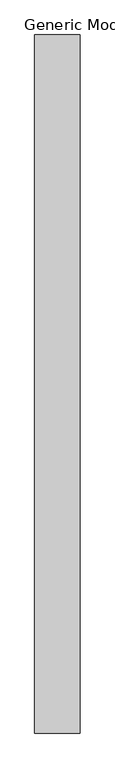
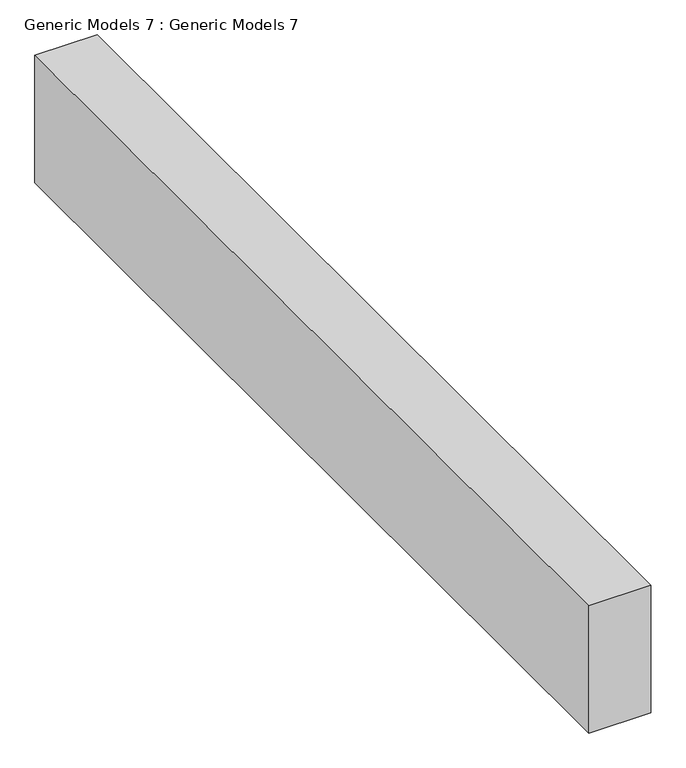
"""IFC4 building model written with IfcOpenShell, lengths in millimetres: proxy geometry, Generic Models 7 : Generic Models 7."""

from ifc_helpers import new_model, si_unit, frame, origin, place, context, project, spatial, polyline, outline, extrude, source, transform, mapped, element, save


def generic_models_7_generic_models_7_1309f326(model_context):
    return source(origin(), model_context, "Body", "SweptSolid", [
        extrude(outline(polyline([(-14730.3406521, -12706.117754), (-14730.3406521, -7997.9810793), (-14425.5406521, -7997.9810793), (-14425.5406521, -12706.117754), (-14730.3406521, -12706.117754)])), frame((0.0, 0.0, 2540.0), z_axis=(0.0, 0.0, 1.0), x_axis=(1.0, 0.0, 0.0)), (0.0, 0.0, 1.0), 660.4),
    ])


if __name__ == "__main__":
    model = new_model("IFC4")
    model_context = context("Model", 3, world=origin())
    ifc_project = project(units=[si_unit("LENGTHUNIT", "METRE", prefix="MILLI")], contexts=[model_context])
    site = spatial("IfcSite", under=ifc_project)
    building = spatial("IfcBuilding", under=site)
    placement = place(None, origin())
    generic_models_7_generic_models_7_shape = generic_models_7_generic_models_7_1309f326(model_context)
    element("IfcBuildingElementProxy", 1, Name="Generic Models 7 : Generic Models 7", ObjectType="Generic Models 7 : Generic Models 7", at=placement, inside=building, context=model_context, shape_type="MappedRepresentation", body=[
        mapped(generic_models_7_generic_models_7_shape, transform((0.0, 0.0, 0.0), x_axis=(1.0, 0.0, 0.0), y_axis=(0.0, 1.0, 0.0), z_axis=(0.0, 0.0, 1.0))),
    ])
    save(model, "model.ifc")

# Revit data of these elements
# Element 1 (IfcBuildingElementProxy, "Generic Models 7 : Generic Models 7")
#   Materials on its faces: "GREY COLOUR FRAME(2)"
# Materials
#   "GREY COLOUR FRAME(2)": class "Generic", colour RGB 120 120 120, transparency 0, Cost = 0
